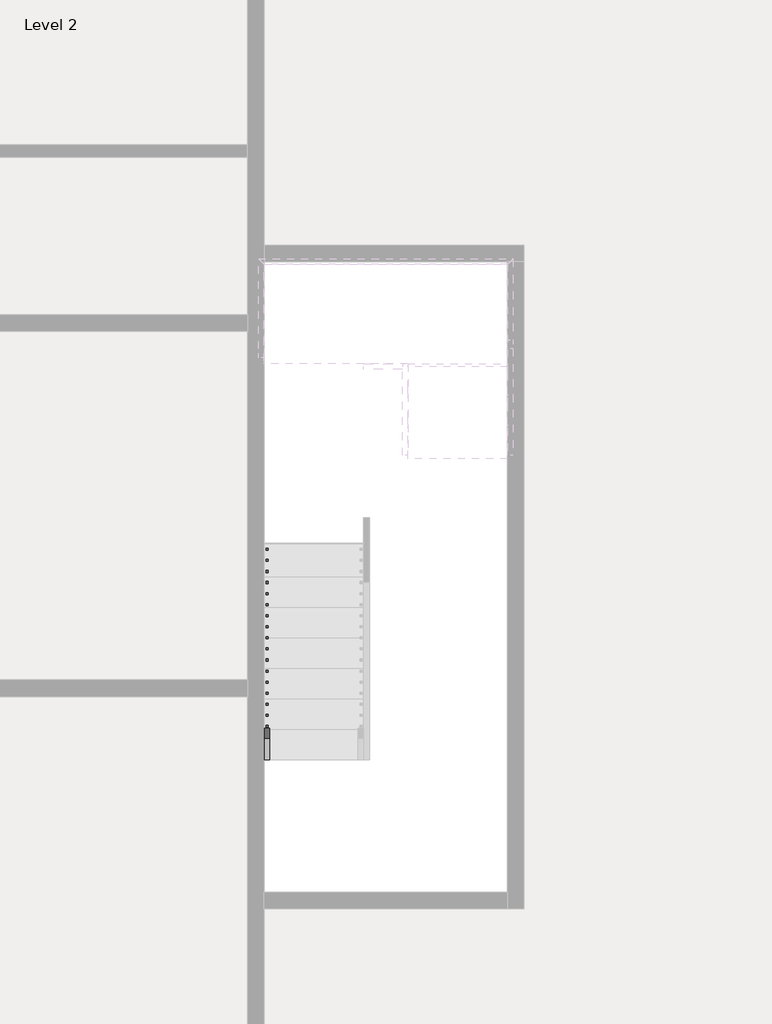
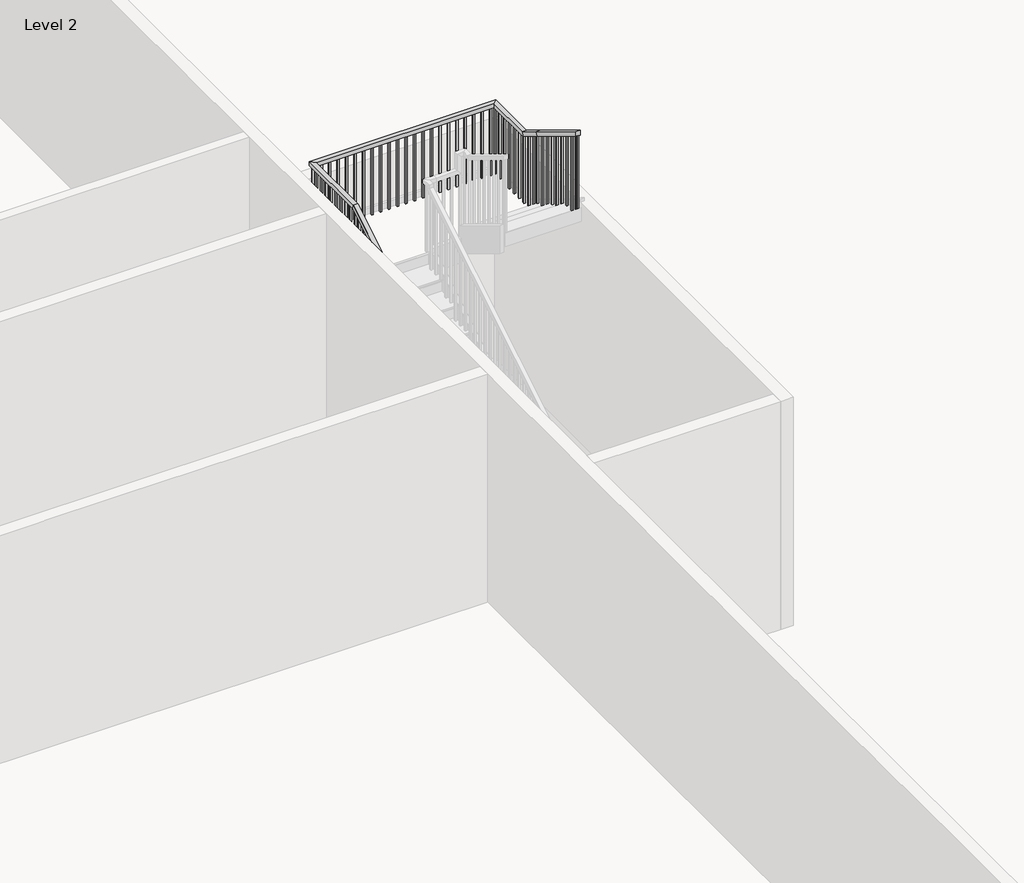
# One storey, part 6 of 8: 1 railing.
"""IFC4 building model written with IfcOpenShell, lengths in millimetres."""

from ifc_helpers import new_model, si_unit, frame, origin, place, context, project, spatial, polyline, outline, extrude, faceted_brep, element, save

model = new_model("IFC4")

# Units and contexts
model_context = context("Model", 3, world=origin())
ifc_project = project(units=[si_unit("LENGTHUNIT", "METRE", prefix="MILLI")], contexts=[model_context])

# Site, building, storey
site = spatial("IfcSite", under=ifc_project)
building = spatial("IfcBuilding", under=site)
storey = spatial("IfcBuildingStorey", under=building, Name="Level 2", Elevation=28282.6172466)

# Railing
placement = place(None, origin())
element("IfcRailing", 1, ObjectType="Handrail - Rectangular", at=placement, inside=storey, context=model_context, shape_type="SolidModel", body=[
    faceted_brep([(-3617.4415084, -23154.3851539, 29366.3505799), (-3617.4415084, -23154.3851539, 29306.9491197), (-3566.6415084, -23154.3851539, 29306.9491197), (-3566.6415084, -23154.3851539, 29366.3505799), (-3617.4415084, -19522.1851539, 31567.6839133), (-3617.4415084, -19507.9927445, 31516.8839133), (-3566.6415084, -19507.9927445, 31516.8839133), (-3566.6415084, -19522.1851539, 31567.6839133), (-3617.4415084, -18607.7851539, 31567.6839133), (-3617.4415084, -18607.7851539, 31516.8839133), (-3566.6415084, -18658.5851539, 31516.8839133), (-3566.6415084, -18658.5851539, 31567.6839133), (-1382.2415084, -18607.7851539, 31567.6839133), (-1382.2415084, -18607.7851539, 31516.8839133), (-1433.0415084, -18658.5851539, 31516.8839133), (-1433.0415084, -18658.5851539, 31567.6839133), (-1382.2415084, -19242.7851539, 31567.6839133), (-1382.2415084, -19256.9775633, 31516.8839133), (-1433.0415084, -19256.9775633, 31516.8839133), (-1433.0415084, -19242.7851539, 31567.6839133), (-1382.2415084, -19522.1851539, 31737.0172466), (-1382.2415084, -19548.5148811, 31693.5731968), (-1433.0415084, -19548.5148811, 31693.5731968), (-1433.0415084, -19522.1851539, 31737.0172466), (-1382.2415084, -20360.3851539, 32245.0172466), (-1433.0415084, -20360.3851539, 32245.0172466), (-1433.0415084, -20360.3851539, 32185.6157863), (-1382.2415084, -20360.3851539, 32185.6157863)], [[[0, 1, 2, 3]], [[1, 0, 4, 5]], [[2, 1, 5, 6]], [[3, 2, 6, 7]], [[0, 3, 7, 4]], [[5, 4, 8, 9]], [[6, 5, 9, 10]], [[7, 6, 10, 11]], [[4, 7, 11, 8]], [[9, 8, 12, 13]], [[10, 9, 13, 14]], [[11, 10, 14, 15]], [[8, 11, 15, 12]], [[13, 12, 16, 17]], [[14, 13, 17, 18]], [[15, 14, 18, 19]], [[12, 15, 19, 16]], [[17, 16, 20, 21]], [[18, 17, 21, 22]], [[19, 18, 22, 23]], [[16, 19, 23, 20]], [[24, 25, 26, 27]], [[21, 20, 24, 27]], [[22, 21, 27, 26]], [[23, 22, 26, 25]], [[20, 23, 25, 24]]]),
    extrude(outline(polyline([(-20325.4601539, 32164.4491197), (-20325.4601539, 31161.2839133), (-20344.5101539, 31161.2839133), (-20344.5101539, 32175.9945742), (-20325.4601539, 32164.4491197)])), frame((-1417.1665084, 0.0, 0.0), z_axis=(1.0, 0.0, 0.0), x_axis=(0.0, 1.0, 0.0)), (0.0, 0.0, 1.0), 19.05),
    extrude(outline(polyline([(-20223.8601539, 32102.8733621), (-20223.8601539, 31161.2839133), (-20242.9101539, 31161.2839133), (-20242.9101539, 32114.4188166), (-20223.8601539, 32102.8733621)])), frame((-1417.1665084, 0.0, 0.0), z_axis=(1.0, 0.0, 0.0), x_axis=(0.0, 1.0, 0.0)), (0.0, 0.0, 1.0), 19.05),
    extrude(outline(polyline([(-20122.2601539, 32041.2976045), (-20122.2601539, 31161.2839133), (-20141.3101539, 31161.2839133), (-20141.3101539, 32052.8430591), (-20122.2601539, 32041.2976045)])), frame((-1417.1665084, 0.0, 0.0), z_axis=(1.0, 0.0, 0.0), x_axis=(0.0, 1.0, 0.0)), (0.0, 0.0, 1.0), 19.05),
    extrude(outline(polyline([(-20020.6601539, 31979.721847), (-20020.6601539, 30991.9505799), (-20039.7101539, 30991.9505799), (-20039.7101539, 31991.2673015), (-20020.6601539, 31979.721847)])), frame((-1417.1665084, 0.0, 0.0), z_axis=(1.0, 0.0, 0.0), x_axis=(0.0, 1.0, 0.0)), (0.0, 0.0, 1.0), 19.05),
    extrude(outline(polyline([(-19919.0601539, 31918.1460894), (-19919.0601539, 30991.9505799), (-19938.1101539, 30991.9505799), (-19938.1101539, 31929.6915439), (-19919.0601539, 31918.1460894)])), frame((-1417.1665084, 0.0, 0.0), z_axis=(1.0, 0.0, 0.0), x_axis=(0.0, 1.0, 0.0)), (0.0, 0.0, 1.0), 19.05),
    extrude(outline(polyline([(-19817.4601539, 31856.5703318), (-19817.4601539, 30991.9505799), (-19836.5101539, 30991.9505799), (-19836.5101539, 31868.1157863), (-19817.4601539, 31856.5703318)])), frame((-1417.1665084, 0.0, 0.0), z_axis=(1.0, 0.0, 0.0), x_axis=(0.0, 1.0, 0.0)), (0.0, 0.0, 1.0), 19.05),
    extrude(outline(polyline([(-19715.8601539, 31794.9945742), (-19715.8601539, 30822.6172466), (-19734.9101539, 30822.6172466), (-19734.9101539, 31806.5400288), (-19715.8601539, 31794.9945742)])), frame((-1417.1665084, 0.0, 0.0), z_axis=(1.0, 0.0, 0.0), x_axis=(0.0, 1.0, 0.0)), (0.0, 0.0, 1.0), 19.05),
    extrude(outline(polyline([(-19614.2601539, 31733.4188166), (-19614.2601539, 30822.6172466), (-19633.3101539, 30822.6172466), (-19633.3101539, 31744.9642712), (-19614.2601539, 31733.4188166)])), frame((-1417.1665084, 0.0, 0.0), z_axis=(1.0, 0.0, 0.0), x_axis=(0.0, 1.0, 0.0)), (0.0, 0.0, 1.0), 19.05),
    extrude(outline(polyline([(-19436.4601539, 31625.6612409), (-19436.4601539, 30653.2839133), (-19455.5101539, 30653.2839133), (-19455.5101539, 31637.2066954), (-19436.4601539, 31625.6612409)])), frame((-1417.1665084, 0.0, 0.0), z_axis=(1.0, 0.0, 0.0), x_axis=(0.0, 1.0, 0.0)), (0.0, 0.0, 1.0), 19.05),
    extrude(outline(polyline([(-19334.8601539, 31564.0854833), (-19334.8601539, 30653.2839133), (-19353.9101539, 30653.2839133), (-19353.9101539, 31575.6309379), (-19334.8601539, 31564.0854833)])), frame((-1417.1665084, 0.0, 0.0), z_axis=(1.0, 0.0, 0.0), x_axis=(0.0, 1.0, 0.0)), (0.0, 0.0, 1.0), 19.05),
    extrude(outline(polyline([(-1398.1165084, -19233.2601539), (-1398.1165084, -19252.3101539), (-1417.1665084, -19252.3101539), (-1417.1665084, -19233.2601539), (-1398.1165084, -19233.2601539)])), frame((0.0, 0.0, 30653.2839133), z_axis=(0.0, 0.0, 1.0), x_axis=(1.0, 0.0, 0.0)), (0.0, 0.0, 1.0), 863.6),
    extrude(outline(polyline([(-1398.1165084, -19131.6601539), (-1398.1165084, -19150.7101539), (-1417.1665084, -19150.7101539), (-1417.1665084, -19131.6601539), (-1398.1165084, -19131.6601539)])), frame((0.0, 0.0, 30653.2839133), z_axis=(0.0, 0.0, 1.0), x_axis=(1.0, 0.0, 0.0)), (0.0, 0.0, 1.0), 863.6),
    extrude(outline(polyline([(-1398.1165084, -19030.0601539), (-1398.1165084, -19049.1101539), (-1417.1665084, -19049.1101539), (-1417.1665084, -19030.0601539), (-1398.1165084, -19030.0601539)])), frame((0.0, 0.0, 30653.2839133), z_axis=(0.0, 0.0, 1.0), x_axis=(1.0, 0.0, 0.0)), (0.0, 0.0, 1.0), 863.6),
    extrude(outline(polyline([(-1398.1165084, -18928.4601539), (-1398.1165084, -18947.5101539), (-1417.1665084, -18947.5101539), (-1417.1665084, -18928.4601539), (-1398.1165084, -18928.4601539)])), frame((0.0, 0.0, 30653.2839133), z_axis=(0.0, 0.0, 1.0), x_axis=(1.0, 0.0, 0.0)), (0.0, 0.0, 1.0), 863.6),
    extrude(outline(polyline([(-1398.1165084, -18826.8601539), (-1398.1165084, -18845.9101539), (-1417.1665084, -18845.9101539), (-1417.1665084, -18826.8601539), (-1398.1165084, -18826.8601539)])), frame((0.0, 0.0, 30653.2839133), z_axis=(0.0, 0.0, 1.0), x_axis=(1.0, 0.0, 0.0)), (0.0, 0.0, 1.0), 863.6),
    extrude(outline(polyline([(-1398.1165084, -18725.2601539), (-1398.1165084, -18744.3101539), (-1417.1665084, -18744.3101539), (-1417.1665084, -18725.2601539), (-1398.1165084, -18725.2601539)])), frame((0.0, 0.0, 30653.2839133), z_axis=(0.0, 0.0, 1.0), x_axis=(1.0, 0.0, 0.0)), (0.0, 0.0, 1.0), 863.6),
    extrude(outline(polyline([(-1467.9665084, -18623.6601539), (-1448.9165084, -18623.6601539), (-1448.9165084, -18642.7101539), (-1467.9665084, -18642.7101539), (-1467.9665084, -18623.6601539)])), frame((0.0, 0.0, 30653.2839133), z_axis=(0.0, 0.0, 1.0), x_axis=(1.0, 0.0, 0.0)), (0.0, 0.0, 1.0), 863.6),
    extrude(outline(polyline([(-1569.5665084, -18623.6601539), (-1550.5165084, -18623.6601539), (-1550.5165084, -18642.7101539), (-1569.5665084, -18642.7101539), (-1569.5665084, -18623.6601539)])), frame((0.0, 0.0, 30653.2839133), z_axis=(0.0, 0.0, 1.0), x_axis=(1.0, 0.0, 0.0)), (0.0, 0.0, 1.0), 863.6),
    extrude(outline(polyline([(-1671.1665084, -18623.6601539), (-1652.1165084, -18623.6601539), (-1652.1165084, -18642.7101539), (-1671.1665084, -18642.7101539), (-1671.1665084, -18623.6601539)])), frame((0.0, 0.0, 30653.2839133), z_axis=(0.0, 0.0, 1.0), x_axis=(1.0, 0.0, 0.0)), (0.0, 0.0, 1.0), 863.6),
    extrude(outline(polyline([(-1772.7665084, -18623.6601539), (-1753.7165084, -18623.6601539), (-1753.7165084, -18642.7101539), (-1772.7665084, -18642.7101539), (-1772.7665084, -18623.6601539)])), frame((0.0, 0.0, 30653.2839133), z_axis=(0.0, 0.0, 1.0), x_axis=(1.0, 0.0, 0.0)), (0.0, 0.0, 1.0), 863.6),
    extrude(outline(polyline([(-1874.3665084, -18623.6601539), (-1855.3165084, -18623.6601539), (-1855.3165084, -18642.7101539), (-1874.3665084, -18642.7101539), (-1874.3665084, -18623.6601539)])), frame((0.0, 0.0, 30653.2839133), z_axis=(0.0, 0.0, 1.0), x_axis=(1.0, 0.0, 0.0)), (0.0, 0.0, 1.0), 863.6),
    extrude(outline(polyline([(-1975.9665084, -18623.6601539), (-1956.9165084, -18623.6601539), (-1956.9165084, -18642.7101539), (-1975.9665084, -18642.7101539), (-1975.9665084, -18623.6601539)])), frame((0.0, 0.0, 30653.2839133), z_axis=(0.0, 0.0, 1.0), x_axis=(1.0, 0.0, 0.0)), (0.0, 0.0, 1.0), 863.6),
    extrude(outline(polyline([(-2077.5665084, -18623.6601539), (-2058.5165084, -18623.6601539), (-2058.5165084, -18642.7101539), (-2077.5665084, -18642.7101539), (-2077.5665084, -18623.6601539)])), frame((0.0, 0.0, 30653.2839133), z_axis=(0.0, 0.0, 1.0), x_axis=(1.0, 0.0, 0.0)), (0.0, 0.0, 1.0), 863.6),
    extrude(outline(polyline([(-2179.1665084, -18623.6601539), (-2160.1165084, -18623.6601539), (-2160.1165084, -18642.7101539), (-2179.1665084, -18642.7101539), (-2179.1665084, -18623.6601539)])), frame((0.0, 0.0, 30653.2839133), z_axis=(0.0, 0.0, 1.0), x_axis=(1.0, 0.0, 0.0)), (0.0, 0.0, 1.0), 863.6),
    extrude(outline(polyline([(-2280.7665084, -18623.6601539), (-2261.7165084, -18623.6601539), (-2261.7165084, -18642.7101539), (-2280.7665084, -18642.7101539), (-2280.7665084, -18623.6601539)])), frame((0.0, 0.0, 30653.2839133), z_axis=(0.0, 0.0, 1.0), x_axis=(1.0, 0.0, 0.0)), (0.0, 0.0, 1.0), 863.6),
    extrude(outline(polyline([(-2382.3665084, -18623.6601539), (-2363.3165084, -18623.6601539), (-2363.3165084, -18642.7101539), (-2382.3665084, -18642.7101539), (-2382.3665084, -18623.6601539)])), frame((0.0, 0.0, 30653.2839133), z_axis=(0.0, 0.0, 1.0), x_axis=(1.0, 0.0, 0.0)), (0.0, 0.0, 1.0), 863.6),
    extrude(outline(polyline([(-2483.9665084, -18623.6601539), (-2464.9165084, -18623.6601539), (-2464.9165084, -18642.7101539), (-2483.9665084, -18642.7101539), (-2483.9665084, -18623.6601539)])), frame((0.0, 0.0, 30653.2839133), z_axis=(0.0, 0.0, 1.0), x_axis=(1.0, 0.0, 0.0)), (0.0, 0.0, 1.0), 863.6),
    extrude(outline(polyline([(-2585.5665084, -18623.6601539), (-2566.5165084, -18623.6601539), (-2566.5165084, -18642.7101539), (-2585.5665084, -18642.7101539), (-2585.5665084, -18623.6601539)])), frame((0.0, 0.0, 30653.2839133), z_axis=(0.0, 0.0, 1.0), x_axis=(1.0, 0.0, 0.0)), (0.0, 0.0, 1.0), 863.6),
    extrude(outline(polyline([(-2687.1665084, -18623.6601539), (-2668.1165084, -18623.6601539), (-2668.1165084, -18642.7101539), (-2687.1665084, -18642.7101539), (-2687.1665084, -18623.6601539)])), frame((0.0, 0.0, 30653.2839133), z_axis=(0.0, 0.0, 1.0), x_axis=(1.0, 0.0, 0.0)), (0.0, 0.0, 1.0), 863.6),
    extrude(outline(polyline([(-2788.7665084, -18623.6601539), (-2769.7165084, -18623.6601539), (-2769.7165084, -18642.7101539), (-2788.7665084, -18642.7101539), (-2788.7665084, -18623.6601539)])), frame((0.0, 0.0, 30653.2839133), z_axis=(0.0, 0.0, 1.0), x_axis=(1.0, 0.0, 0.0)), (0.0, 0.0, 1.0), 863.6),
    extrude(outline(polyline([(-2890.3665084, -18623.6601539), (-2871.3165084, -18623.6601539), (-2871.3165084, -18642.7101539), (-2890.3665084, -18642.7101539), (-2890.3665084, -18623.6601539)])), frame((0.0, 0.0, 30653.2839133), z_axis=(0.0, 0.0, 1.0), x_axis=(1.0, 0.0, 0.0)), (0.0, 0.0, 1.0), 863.6),
    extrude(outline(polyline([(-2991.9665084, -18623.6601539), (-2972.9165084, -18623.6601539), (-2972.9165084, -18642.7101539), (-2991.9665084, -18642.7101539), (-2991.9665084, -18623.6601539)])), frame((0.0, 0.0, 30653.2839133), z_axis=(0.0, 0.0, 1.0), x_axis=(1.0, 0.0, 0.0)), (0.0, 0.0, 1.0), 863.6),
    extrude(outline(polyline([(-3093.5665084, -18623.6601539), (-3074.5165084, -18623.6601539), (-3074.5165084, -18642.7101539), (-3093.5665084, -18642.7101539), (-3093.5665084, -18623.6601539)])), frame((0.0, 0.0, 30653.2839133), z_axis=(0.0, 0.0, 1.0), x_axis=(1.0, 0.0, 0.0)), (0.0, 0.0, 1.0), 863.6),
    extrude(outline(polyline([(-3195.1665084, -18623.6601539), (-3176.1165084, -18623.6601539), (-3176.1165084, -18642.7101539), (-3195.1665084, -18642.7101539), (-3195.1665084, -18623.6601539)])), frame((0.0, 0.0, 30653.2839133), z_axis=(0.0, 0.0, 1.0), x_axis=(1.0, 0.0, 0.0)), (0.0, 0.0, 1.0), 863.6),
    extrude(outline(polyline([(-3296.7665084, -18623.6601539), (-3277.7165084, -18623.6601539), (-3277.7165084, -18642.7101539), (-3296.7665084, -18642.7101539), (-3296.7665084, -18623.6601539)])), frame((0.0, 0.0, 30653.2839133), z_axis=(0.0, 0.0, 1.0), x_axis=(1.0, 0.0, 0.0)), (0.0, 0.0, 1.0), 863.6),
    extrude(outline(polyline([(-3398.3665084, -18623.6601539), (-3379.3165084, -18623.6601539), (-3379.3165084, -18642.7101539), (-3398.3665084, -18642.7101539), (-3398.3665084, -18623.6601539)])), frame((0.0, 0.0, 30653.2839133), z_axis=(0.0, 0.0, 1.0), x_axis=(1.0, 0.0, 0.0)), (0.0, 0.0, 1.0), 863.6),
    extrude(outline(polyline([(-3499.9665084, -18623.6601539), (-3480.9165084, -18623.6601539), (-3480.9165084, -18642.7101539), (-3499.9665084, -18642.7101539), (-3499.9665084, -18623.6601539)])), frame((0.0, 0.0, 30653.2839133), z_axis=(0.0, 0.0, 1.0), x_axis=(1.0, 0.0, 0.0)), (0.0, 0.0, 1.0), 863.6),
    extrude(outline(polyline([(-3601.5665084, -18718.9101539), (-3601.5665084, -18699.8601539), (-3582.5165084, -18699.8601539), (-3582.5165084, -18718.9101539), (-3601.5665084, -18718.9101539)])), frame((0.0, 0.0, 30653.2839133), z_axis=(0.0, 0.0, 1.0), x_axis=(1.0, 0.0, 0.0)), (0.0, 0.0, 1.0), 863.6),
    extrude(outline(polyline([(-3601.5665084, -18820.5101539), (-3601.5665084, -18801.4601539), (-3582.5165084, -18801.4601539), (-3582.5165084, -18820.5101539), (-3601.5665084, -18820.5101539)])), frame((0.0, 0.0, 30653.2839133), z_axis=(0.0, 0.0, 1.0), x_axis=(1.0, 0.0, 0.0)), (0.0, 0.0, 1.0), 863.6),
    extrude(outline(polyline([(-3601.5665084, -18922.1101539), (-3601.5665084, -18903.0601539), (-3582.5165084, -18903.0601539), (-3582.5165084, -18922.1101539), (-3601.5665084, -18922.1101539)])), frame((0.0, 0.0, 30653.2839133), z_axis=(0.0, 0.0, 1.0), x_axis=(1.0, 0.0, 0.0)), (0.0, 0.0, 1.0), 863.6),
    extrude(outline(polyline([(-3601.5665084, -19023.7101539), (-3601.5665084, -19004.6601539), (-3582.5165084, -19004.6601539), (-3582.5165084, -19023.7101539), (-3601.5665084, -19023.7101539)])), frame((0.0, 0.0, 30653.2839133), z_axis=(0.0, 0.0, 1.0), x_axis=(1.0, 0.0, 0.0)), (0.0, 0.0, 1.0), 863.6),
    extrude(outline(polyline([(-3601.5665084, -19125.3101539), (-3601.5665084, -19106.2601539), (-3582.5165084, -19106.2601539), (-3582.5165084, -19125.3101539), (-3601.5665084, -19125.3101539)])), frame((0.0, 0.0, 30653.2839133), z_axis=(0.0, 0.0, 1.0), x_axis=(1.0, 0.0, 0.0)), (0.0, 0.0, 1.0), 863.6),
    extrude(outline(polyline([(-3601.5665084, -19226.9101539), (-3601.5665084, -19207.8601539), (-3582.5165084, -19207.8601539), (-3582.5165084, -19226.9101539), (-3601.5665084, -19226.9101539)])), frame((0.0, 0.0, 30653.2839133), z_axis=(0.0, 0.0, 1.0), x_axis=(1.0, 0.0, 0.0)), (0.0, 0.0, 1.0), 863.6),
    extrude(outline(polyline([(-3601.5665084, -19328.5101539), (-3601.5665084, -19309.4601539), (-3582.5165084, -19309.4601539), (-3582.5165084, -19328.5101539), (-3601.5665084, -19328.5101539)])), frame((0.0, 0.0, 30653.2839133), z_axis=(0.0, 0.0, 1.0), x_axis=(1.0, 0.0, 0.0)), (0.0, 0.0, 1.0), 863.6),
    extrude(outline(polyline([(-3601.5665084, -19430.1101539), (-3601.5665084, -19411.0601539), (-3582.5165084, -19411.0601539), (-3582.5165084, -19430.1101539), (-3601.5665084, -19430.1101539)])), frame((0.0, 0.0, 30653.2839133), z_axis=(0.0, 0.0, 1.0), x_axis=(1.0, 0.0, 0.0)), (0.0, 0.0, 1.0), 863.6),
    extrude(outline(polyline([(-19588.8601539, 31467.8733621), (-19588.8601539, 30483.9505799), (-19607.9101539, 30483.9505799), (-19607.9101539, 31456.3279076), (-19588.8601539, 31467.8733621)])), frame((-3601.5665084, 0.0, 0.0), z_axis=(1.0, 0.0, 0.0), x_axis=(0.0, 1.0, 0.0)), (0.0, 0.0, 1.0), 19.05),
    extrude(outline(polyline([(-19690.4601539, 31406.2976045), (-19690.4601539, 30483.9505799), (-19709.5101539, 30483.9505799), (-19709.5101539, 31394.75215), (-19690.4601539, 31406.2976045)])), frame((-3601.5665084, 0.0, 0.0), z_axis=(1.0, 0.0, 0.0), x_axis=(0.0, 1.0, 0.0)), (0.0, 0.0, 1.0), 19.05),
    extrude(outline(polyline([(-19792.0601539, 31344.721847), (-19792.0601539, 30483.9505799), (-19811.1101539, 30483.9505799), (-19811.1101539, 31333.1763924), (-19792.0601539, 31344.721847)])), frame((-3601.5665084, 0.0, 0.0), z_axis=(1.0, 0.0, 0.0), x_axis=(0.0, 1.0, 0.0)), (0.0, 0.0, 1.0), 19.05),
    extrude(outline(polyline([(-19893.6601539, 31283.1460894), (-19893.6601539, 30314.6172466), (-19912.7101539, 30314.6172466), (-19912.7101539, 31271.6006348), (-19893.6601539, 31283.1460894)])), frame((-3601.5665084, 0.0, 0.0), z_axis=(1.0, 0.0, 0.0), x_axis=(0.0, 1.0, 0.0)), (0.0, 0.0, 1.0), 19.05),
    extrude(outline(polyline([(-19995.2601539, 31221.5703318), (-19995.2601539, 30314.6172466), (-20014.3101539, 30314.6172466), (-20014.3101539, 31210.0248773), (-19995.2601539, 31221.5703318)])), frame((-3601.5665084, 0.0, 0.0), z_axis=(1.0, 0.0, 0.0), x_axis=(0.0, 1.0, 0.0)), (0.0, 0.0, 1.0), 19.05),
    extrude(outline(polyline([(-20096.8601539, 31159.9945742), (-20096.8601539, 30145.2839133), (-20115.9101539, 30145.2839133), (-20115.9101539, 31148.4491197), (-20096.8601539, 31159.9945742)])), frame((-3601.5665084, 0.0, 0.0), z_axis=(1.0, 0.0, 0.0), x_axis=(0.0, 1.0, 0.0)), (0.0, 0.0, 1.0), 19.05),
    extrude(outline(polyline([(-20198.4601539, 31098.4188167), (-20198.4601539, 30145.2839133), (-20217.5101539, 30145.2839133), (-20217.5101539, 31086.8733621), (-20198.4601539, 31098.4188167)])), frame((-3601.5665084, 0.0, 0.0), z_axis=(1.0, 0.0, 0.0), x_axis=(0.0, 1.0, 0.0)), (0.0, 0.0, 1.0), 19.05),
    extrude(outline(polyline([(-20300.0601539, 31036.8430591), (-20300.0601539, 30145.2839133), (-20319.1101539, 30145.2839133), (-20319.1101539, 31025.2976045), (-20300.0601539, 31036.8430591)])), frame((-3601.5665084, 0.0, 0.0), z_axis=(1.0, 0.0, 0.0), x_axis=(0.0, 1.0, 0.0)), (0.0, 0.0, 1.0), 19.05),
    extrude(outline(polyline([(-20401.6601539, 30975.2673015), (-20401.6601539, 29975.9505799), (-20420.7101539, 29975.9505799), (-20420.7101539, 30963.721847), (-20401.6601539, 30975.2673015)])), frame((-3601.5665084, 0.0, 0.0), z_axis=(1.0, 0.0, 0.0), x_axis=(0.0, 1.0, 0.0)), (0.0, 0.0, 1.0), 19.05),
    extrude(outline(polyline([(-20503.2601539, 30913.6915439), (-20503.2601539, 29975.9505799), (-20522.3101539, 29975.9505799), (-20522.3101539, 30902.1460894), (-20503.2601539, 30913.6915439)])), frame((-3601.5665084, 0.0, 0.0), z_axis=(1.0, 0.0, 0.0), x_axis=(0.0, 1.0, 0.0)), (0.0, 0.0, 1.0), 19.05),
    extrude(outline(polyline([(-20604.8601539, 30852.1157863), (-20604.8601539, 29975.9505799), (-20623.9101539, 29975.9505799), (-20623.9101539, 30840.5703318), (-20604.8601539, 30852.1157863)])), frame((-3601.5665084, 0.0, 0.0), z_axis=(1.0, 0.0, 0.0), x_axis=(0.0, 1.0, 0.0)), (0.0, 0.0, 1.0), 19.05),
    extrude(outline(polyline([(-20706.4601539, 30790.5400288), (-20706.4601539, 29806.6172466), (-20725.5101539, 29806.6172466), (-20725.5101539, 30778.9945742), (-20706.4601539, 30790.5400288)])), frame((-3601.5665084, 0.0, 0.0), z_axis=(1.0, 0.0, 0.0), x_axis=(0.0, 1.0, 0.0)), (0.0, 0.0, 1.0), 19.05),
    extrude(outline(polyline([(-20808.0601539, 30728.9642712), (-20808.0601539, 29806.6172466), (-20827.1101539, 29806.6172466), (-20827.1101539, 30717.4188167), (-20808.0601539, 30728.9642712)])), frame((-3601.5665084, 0.0, 0.0), z_axis=(1.0, 0.0, 0.0), x_axis=(0.0, 1.0, 0.0)), (0.0, 0.0, 1.0), 19.05),
    extrude(outline(polyline([(-20909.6601539, 30667.3885136), (-20909.6601539, 29806.6172466), (-20928.7101539, 29806.6172466), (-20928.7101539, 30655.8430591), (-20909.6601539, 30667.3885136)])), frame((-3601.5665084, 0.0, 0.0), z_axis=(1.0, 0.0, 0.0), x_axis=(0.0, 1.0, 0.0)), (0.0, 0.0, 1.0), 19.05),
    extrude(outline(polyline([(-21011.2601539, 30605.812756), (-21011.2601539, 29637.2839133), (-21030.3101539, 29637.2839133), (-21030.3101539, 30594.2673015), (-21011.2601539, 30605.812756)])), frame((-3601.5665084, 0.0, 0.0), z_axis=(1.0, 0.0, 0.0), x_axis=(0.0, 1.0, 0.0)), (0.0, 0.0, 1.0), 19.05),
    extrude(outline(polyline([(-21112.8601539, 30544.2369985), (-21112.8601539, 29637.2839133), (-21131.9101539, 29637.2839133), (-21131.9101539, 30532.6915439), (-21112.8601539, 30544.2369985)])), frame((-3601.5665084, 0.0, 0.0), z_axis=(1.0, 0.0, 0.0), x_axis=(0.0, 1.0, 0.0)), (0.0, 0.0, 1.0), 19.05),
    extrude(outline(polyline([(-21214.4601539, 30482.6612409), (-21214.4601539, 29467.9505799), (-21233.5101539, 29467.9505799), (-21233.5101539, 30471.1157863), (-21214.4601539, 30482.6612409)])), frame((-3601.5665084, 0.0, 0.0), z_axis=(1.0, 0.0, 0.0), x_axis=(0.0, 1.0, 0.0)), (0.0, 0.0, 1.0), 19.05),
    extrude(outline(polyline([(-21316.0601539, 30421.0854833), (-21316.0601539, 29467.9505799), (-21335.1101539, 29467.9505799), (-21335.1101539, 30409.5400288), (-21316.0601539, 30421.0854833)])), frame((-3601.5665084, 0.0, 0.0), z_axis=(1.0, 0.0, 0.0), x_axis=(0.0, 1.0, 0.0)), (0.0, 0.0, 1.0), 19.05),
    extrude(outline(polyline([(-21417.6601539, 30359.5097257), (-21417.6601539, 29467.9505799), (-21436.7101539, 29467.9505799), (-21436.7101539, 30347.9642712), (-21417.6601539, 30359.5097257)])), frame((-3601.5665084, 0.0, 0.0), z_axis=(1.0, 0.0, 0.0), x_axis=(0.0, 1.0, 0.0)), (0.0, 0.0, 1.0), 19.05),
    extrude(outline(polyline([(-21519.2601539, 30297.9339682), (-21519.2601539, 29298.6172466), (-21538.3101539, 29298.6172466), (-21538.3101539, 30286.3885136), (-21519.2601539, 30297.9339682)])), frame((-3601.5665084, 0.0, 0.0), z_axis=(1.0, 0.0, 0.0), x_axis=(0.0, 1.0, 0.0)), (0.0, 0.0, 1.0), 19.05),
    extrude(outline(polyline([(-21620.8601539, 30236.3582106), (-21620.8601539, 29298.6172466), (-21639.9101539, 29298.6172466), (-21639.9101539, 30224.812756), (-21620.8601539, 30236.3582106)])), frame((-3601.5665084, 0.0, 0.0), z_axis=(1.0, 0.0, 0.0), x_axis=(0.0, 1.0, 0.0)), (0.0, 0.0, 1.0), 19.05),
    extrude(outline(polyline([(-21722.4601539, 30174.782453), (-21722.4601539, 29298.6172466), (-21741.5101539, 29298.6172466), (-21741.5101539, 30163.2369985), (-21722.4601539, 30174.782453)])), frame((-3601.5665084, 0.0, 0.0), z_axis=(1.0, 0.0, 0.0), x_axis=(0.0, 1.0, 0.0)), (0.0, 0.0, 1.0), 19.05),
    extrude(outline(polyline([(-21824.0601539, 30113.2066954), (-21824.0601539, 29129.2839133), (-21843.1101539, 29129.2839133), (-21843.1101539, 30101.6612409), (-21824.0601539, 30113.2066954)])), frame((-3601.5665084, 0.0, 0.0), z_axis=(1.0, 0.0, 0.0), x_axis=(0.0, 1.0, 0.0)), (0.0, 0.0, 1.0), 19.05),
    extrude(outline(polyline([(-21925.6601539, 30051.6309379), (-21925.6601539, 29129.2839133), (-21944.7101539, 29129.2839133), (-21944.7101539, 30040.0854833), (-21925.6601539, 30051.6309379)])), frame((-3601.5665084, 0.0, 0.0), z_axis=(1.0, 0.0, 0.0), x_axis=(0.0, 1.0, 0.0)), (0.0, 0.0, 1.0), 19.05),
    extrude(outline(polyline([(-22027.2601539, 29990.0551803), (-22027.2601539, 29129.2839133), (-22046.3101539, 29129.2839133), (-22046.3101539, 29978.5097257), (-22027.2601539, 29990.0551803)])), frame((-3601.5665084, 0.0, 0.0), z_axis=(1.0, 0.0, 0.0), x_axis=(0.0, 1.0, 0.0)), (0.0, 0.0, 1.0), 19.05),
    extrude(outline(polyline([(-22128.8601539, 29928.4794227), (-22128.8601539, 28959.9505799), (-22147.9101539, 28959.9505799), (-22147.9101539, 29916.9339682), (-22128.8601539, 29928.4794227)])), frame((-3601.5665084, 0.0, 0.0), z_axis=(1.0, 0.0, 0.0), x_axis=(0.0, 1.0, 0.0)), (0.0, 0.0, 1.0), 19.05),
    extrude(outline(polyline([(-22230.4601539, 29866.9036651), (-22230.4601539, 28959.9505799), (-22249.5101539, 28959.9505799), (-22249.5101539, 29855.3582106), (-22230.4601539, 29866.9036651)])), frame((-3601.5665084, 0.0, 0.0), z_axis=(1.0, 0.0, 0.0), x_axis=(0.0, 1.0, 0.0)), (0.0, 0.0, 1.0), 19.05),
    extrude(outline(polyline([(-22332.0601539, 29805.3279076), (-22332.0601539, 28790.6172466), (-22351.1101539, 28790.6172466), (-22351.1101539, 29793.782453), (-22332.0601539, 29805.3279076)])), frame((-3601.5665084, 0.0, 0.0), z_axis=(1.0, 0.0, 0.0), x_axis=(0.0, 1.0, 0.0)), (0.0, 0.0, 1.0), 19.05),
    extrude(outline(polyline([(-22433.6601539, 29743.75215), (-22433.6601539, 28790.6172466), (-22452.7101539, 28790.6172466), (-22452.7101539, 29732.2066954), (-22433.6601539, 29743.75215)])), frame((-3601.5665084, 0.0, 0.0), z_axis=(1.0, 0.0, 0.0), x_axis=(0.0, 1.0, 0.0)), (0.0, 0.0, 1.0), 19.05),
    extrude(outline(polyline([(-22535.2601539, 29682.1763924), (-22535.2601539, 28790.6172466), (-22554.3101539, 28790.6172466), (-22554.3101539, 29670.6309379), (-22535.2601539, 29682.1763924)])), frame((-3601.5665084, 0.0, 0.0), z_axis=(1.0, 0.0, 0.0), x_axis=(0.0, 1.0, 0.0)), (0.0, 0.0, 1.0), 19.05),
    extrude(outline(polyline([(-22636.8601539, 29620.6006348), (-22636.8601539, 28621.2839133), (-22655.9101539, 28621.2839133), (-22655.9101539, 29609.0551803), (-22636.8601539, 29620.6006348)])), frame((-3601.5665084, 0.0, 0.0), z_axis=(1.0, 0.0, 0.0), x_axis=(0.0, 1.0, 0.0)), (0.0, 0.0, 1.0), 19.05),
    extrude(outline(polyline([(-22738.4601539, 29559.0248773), (-22738.4601539, 28621.2839133), (-22757.5101539, 28621.2839133), (-22757.5101539, 29547.4794227), (-22738.4601539, 29559.0248773)])), frame((-3601.5665084, 0.0, 0.0), z_axis=(1.0, 0.0, 0.0), x_axis=(0.0, 1.0, 0.0)), (0.0, 0.0, 1.0), 19.05),
    extrude(outline(polyline([(-22840.0601539, 29497.4491197), (-22840.0601539, 28621.2839133), (-22859.1101539, 28621.2839133), (-22859.1101539, 29485.9036651), (-22840.0601539, 29497.4491197)])), frame((-3601.5665084, 0.0, 0.0), z_axis=(1.0, 0.0, 0.0), x_axis=(0.0, 1.0, 0.0)), (0.0, 0.0, 1.0), 19.05),
    extrude(outline(polyline([(-22941.6601539, 29435.8733621), (-22941.6601539, 28451.9505799), (-22960.7101539, 28451.9505799), (-22960.7101539, 29424.3279076), (-22941.6601539, 29435.8733621)])), frame((-3601.5665084, 0.0, 0.0), z_axis=(1.0, 0.0, 0.0), x_axis=(0.0, 1.0, 0.0)), (0.0, 0.0, 1.0), 19.05),
    extrude(outline(polyline([(-23043.2601539, 29374.2976045), (-23043.2601539, 28451.9505799), (-23062.3101539, 28451.9505799), (-23062.3101539, 29362.75215), (-23043.2601539, 29374.2976045)])), frame((-3601.5665084, 0.0, 0.0), z_axis=(1.0, 0.0, 0.0), x_axis=(0.0, 1.0, 0.0)), (0.0, 0.0, 1.0), 19.05),
    extrude(outline(polyline([(-19512.6601539, 31671.8430591), (-19512.6601539, 30653.2839133), (-19531.7101539, 30653.2839133), (-19531.7101539, 31683.3885136), (-19512.6601539, 31671.8430591)])), frame((-1417.1665084, 0.0, 0.0), z_axis=(1.0, 0.0, 0.0), x_axis=(0.0, 1.0, 0.0)), (0.0, 0.0, 1.0), 19.05),
    extrude(outline(polyline([(-1417.1665084, -18623.6601539), (-1398.1165084, -18623.6601539), (-1398.1165084, -18642.7101539), (-1417.1665084, -18642.7101539), (-1417.1665084, -18623.6601539)])), frame((0.0, 0.0, 30653.2839133), z_axis=(0.0, 0.0, 1.0), x_axis=(1.0, 0.0, 0.0)), (0.0, 0.0, 1.0), 863.6),
    extrude(outline(polyline([(-3601.5665084, -18642.7101539), (-3601.5665084, -18623.6601539), (-3582.5165084, -18623.6601539), (-3582.5165084, -18642.7101539), (-3601.5665084, -18642.7101539)])), frame((0.0, 0.0, 30653.2839133), z_axis=(0.0, 0.0, 1.0), x_axis=(1.0, 0.0, 0.0)), (0.0, 0.0, 1.0), 863.6),
    extrude(outline(polyline([(-19512.6601539, 31514.0551803), (-19512.6601539, 30653.2839133), (-19531.7101539, 30653.2839133), (-19531.7101539, 31502.5097257), (-19512.6601539, 31514.0551803)])), frame((-3601.5665084, 0.0, 0.0), z_axis=(1.0, 0.0, 0.0), x_axis=(0.0, 1.0, 0.0)), (0.0, 0.0, 1.0), 19.05),
    extrude(outline(polyline([(-20341.3351539, 32174.0703318), (-20341.3351539, 31161.2839133), (-20360.3851539, 31161.2839133), (-20360.3851539, 32185.6157863), (-20341.3351539, 32174.0703318)])), frame((-1417.1665084, 0.0, 0.0), z_axis=(1.0, 0.0, 0.0), x_axis=(0.0, 1.0, 0.0)), (0.0, 0.0, 1.0), 19.05),
    extrude(outline(polyline([(-23135.3351539, 29318.4945742), (-23135.3351539, 28451.9505799), (-23154.3851539, 28451.9505799), (-23154.3851539, 29306.9491197), (-23135.3351539, 29318.4945742)])), frame((-3601.5665084, 0.0, 0.0), z_axis=(1.0, 0.0, 0.0), x_axis=(0.0, 1.0, 0.0)), (0.0, 0.0, 1.0), 19.05),
])

save(model, "model.ifc")

# Revit data of these elements
# Type "Handrail - Rectangular"
#   Assembly Code = "C2010400"
#   built-in parameter 1008612 = 0.0416667 (stored number, unit not read)
#   built-in parameter 1008611 = 0.0416667 (stored number, unit not read)
#   built-in parameter 1008609 = 0.333333 (stored number, unit not read)
#   built-in parameter 1008604 = 0.166667 (stored number, unit not read)
#   built-in parameter 1008603 = 0.166667 (stored number, unit not read)
#   Railing Height = 3' - 0"
#   built-in parameter 1008630 = 2
#   built-in parameter 1008610 = 2
#   built-in parameter 1008618 = Baluster - Square : 3/4"
# Element 1 (IfcRailing, "Handrail - Rectangular")
#   Phase Created = New Construction
